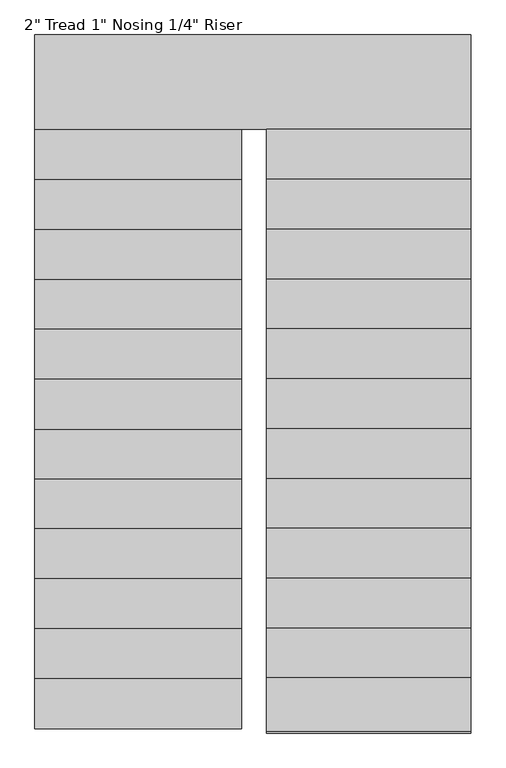
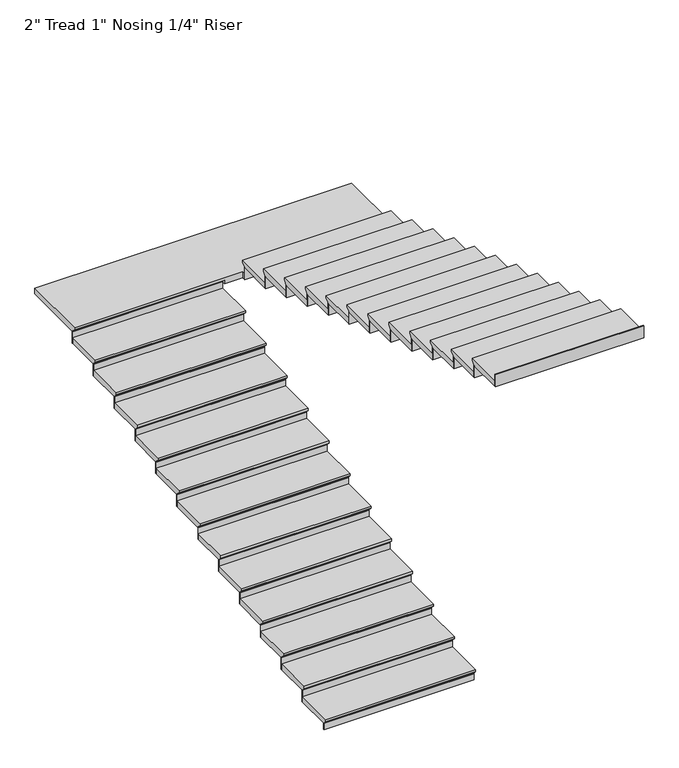
"""IFC4 building model written with IfcOpenShell, lengths in millimetres: stair flight geometry."""

from ifc_helpers import new_model, si_unit, origin, place, context, project, spatial, faceted_brep, source, transform, mapped, element, save


def stair_flight_04159850(model_context):
    return source(origin(), model_context, "Body", "Brep", [
        faceted_brep([(-2593.7381751, -9955.5916506, 12278.4576923), (-2593.7381751, -9955.5916506, 12297.5076923), (-3857.687215, -9955.5916506, 12297.5076923), (-3857.687215, -9955.5916506, 12278.4576923), (-2593.7381751, -9930.1916506, 12253.0576923), (-3857.687215, -9930.1916506, 12253.0576923), (-2593.7381751, -9619.0416506, 12297.5076923), (-3857.687215, -9619.0416506, 12297.5076923), (-3857.687215, -9930.1916506, 12246.7076923), (-3857.687215, -9619.0416506, 12246.7076923), (-2593.7381751, -9619.0416506, 12246.7076923), (-2593.7381751, -9930.1916506, 12246.7076923)], [[[0, 1, 2, 3]], [[4, 0, 3, 5]], [[2, 1, 6, 7]], [[8, 9, 10, 11]], [[2, 7, 9, 8, 5, 3]], [[8, 11, 4, 5]], [[6, 1, 0, 4, 11, 10]], [[7, 6, 10, 9]]]),
        faceted_brep([(-2593.7381751, -9930.1916506, 12246.7076923), (-2593.7381751, -9930.1916506, 12192.0), (-2593.7381751, -9923.8416506, 12192.0), (-2593.7381751, -9923.8416506, 12246.7076923), (-3857.687215, -9930.1916506, 12246.7076923), (-3857.687215, -9923.8416506, 12246.7076923), (-3857.687215, -9923.8416506, 12192.0), (-3857.687215, -9930.1916506, 12192.0)], [[[0, 1, 2, 3]], [[4, 5, 6, 7]], [[1, 0, 4, 7]], [[2, 1, 7, 6]], [[3, 2, 6, 5]], [[0, 3, 5, 4]]]),
        faceted_brep([(-2593.7381751, -9619.0416506, 12352.2153846), (-2593.7381751, -9619.0416506, 12246.7076923), (-2593.7381751, -9612.6916506, 12246.7076923), (-2593.7381751, -9612.6916506, 12352.2153846), (-3857.687215, -9619.0416506, 12352.2153846), (-3857.687215, -9612.6916506, 12352.2153846), (-3857.687215, -9612.6916506, 12246.7076923), (-3857.687215, -9619.0416506, 12246.7076923)], [[[0, 1, 2, 3]], [[4, 5, 6, 7]], [[1, 0, 4, 7]], [[2, 1, 7, 6]], [[3, 2, 6, 5]], [[0, 3, 5, 4]]]),
        faceted_brep([(-3857.687215, -9644.4416506, 12403.0153846), (-2593.7381751, -9644.4416506, 12403.0153846), (-2593.7381751, -9314.2416506, 12403.0153846), (-3857.687215, -9314.2416506, 12403.0153846), (-3857.687215, -9619.0416506, 12352.2153846), (-3857.687215, -9314.2416506, 12352.2153846), (-2593.7381751, -9314.2416506, 12352.2153846), (-2593.7381751, -9619.0416506, 12352.2153846), (-3857.687215, -9619.0416506, 12358.5653846), (-3857.687215, -9644.4416506, 12383.9653846), (-2593.7381751, -9619.0416506, 12358.5653846), (-2593.7381751, -9644.4416506, 12383.9653846)], [[[0, 1, 2, 3]], [[4, 5, 6, 7]], [[0, 3, 5, 4, 8, 9]], [[4, 7, 10, 8]], [[2, 1, 11, 10, 7, 6]], [[3, 2, 6, 5]], [[11, 1, 0, 9]], [[10, 11, 9, 8]]]),
        faceted_brep([(-2593.7381751, -9314.2416506, 12457.7230769), (-2593.7381751, -9314.2416506, 12352.2153846), (-2593.7381751, -9307.8916506, 12352.2153846), (-2593.7381751, -9307.8916506, 12457.7230769), (-3857.687215, -9314.2416506, 12457.7230769), (-3857.687215, -9307.8916506, 12457.7230769), (-3857.687215, -9307.8916506, 12352.2153846), (-3857.687215, -9314.2416506, 12352.2153846)], [[[0, 1, 2, 3]], [[4, 5, 6, 7]], [[1, 0, 4, 7]], [[2, 1, 7, 6]], [[3, 2, 6, 5]], [[0, 3, 5, 4]]]),
        faceted_brep([(-3857.687215, -9339.6416506, 12508.5230769), (-2593.7381751, -9339.6416506, 12508.5230769), (-2593.7381751, -9009.4416506, 12508.5230769), (-3857.687215, -9009.4416506, 12508.5230769), (-3857.687215, -9314.2416506, 12457.7230769), (-3857.687215, -9009.4416506, 12457.7230769), (-2593.7381751, -9009.4416506, 12457.7230769), (-2593.7381751, -9314.2416506, 12457.7230769), (-3857.687215, -9314.2416506, 12464.0730769), (-3857.687215, -9339.6416506, 12489.4730769), (-2593.7381751, -9314.2416506, 12464.0730769), (-2593.7381751, -9339.6416506, 12489.4730769)], [[[0, 1, 2, 3]], [[4, 5, 6, 7]], [[0, 3, 5, 4, 8, 9]], [[4, 7, 10, 8]], [[2, 1, 11, 10, 7, 6]], [[3, 2, 6, 5]], [[11, 1, 0, 9]], [[10, 11, 9, 8]]]),
        faceted_brep([(-2593.7381751, -9009.4416506, 12563.2307692), (-2593.7381751, -9009.4416506, 12457.7230769), (-2593.7381751, -9003.0916506, 12457.7230769), (-2593.7381751, -9003.0916506, 12563.2307692), (-3857.687215, -9009.4416506, 12563.2307692), (-3857.687215, -9003.0916506, 12563.2307692), (-3857.687215, -9003.0916506, 12457.7230769), (-3857.687215, -9009.4416506, 12457.7230769)], [[[0, 1, 2, 3]], [[4, 5, 6, 7]], [[1, 0, 4, 7]], [[2, 1, 7, 6]], [[3, 2, 6, 5]], [[0, 3, 5, 4]]]),
        faceted_brep([(-3857.687215, -9034.8416506, 12614.0307692), (-2593.7381751, -9034.8416506, 12614.0307692), (-2593.7381751, -8704.6416506, 12614.0307692), (-3857.687215, -8704.6416506, 12614.0307692), (-3857.687215, -9009.4416506, 12563.2307692), (-3857.687215, -8704.6416506, 12563.2307692), (-2593.7381751, -8704.6416506, 12563.2307692), (-2593.7381751, -9009.4416506, 12563.2307692), (-3857.687215, -9009.4416506, 12569.5807692), (-3857.687215, -9034.8416506, 12594.9807692), (-2593.7381751, -9009.4416506, 12569.5807692), (-2593.7381751, -9034.8416506, 12594.9807692)], [[[0, 1, 2, 3]], [[4, 5, 6, 7]], [[0, 3, 5, 4, 8, 9]], [[4, 7, 10, 8]], [[2, 1, 11, 10, 7, 6]], [[3, 2, 6, 5]], [[11, 1, 0, 9]], [[10, 11, 9, 8]]]),
        faceted_brep([(-2593.7381751, -8704.6416506, 12668.7384615), (-2593.7381751, -8704.6416506, 12563.2307692), (-2593.7381751, -8698.2916506, 12563.2307692), (-2593.7381751, -8698.2916506, 12668.7384615), (-3857.687215, -8704.6416506, 12668.7384615), (-3857.687215, -8698.2916506, 12668.7384615), (-3857.687215, -8698.2916506, 12563.2307692), (-3857.687215, -8704.6416506, 12563.2307692)], [[[0, 1, 2, 3]], [[4, 5, 6, 7]], [[1, 0, 4, 7]], [[2, 1, 7, 6]], [[3, 2, 6, 5]], [[0, 3, 5, 4]]]),
        faceted_brep([(-3857.687215, -8730.0416506, 12719.5384615), (-2593.7381751, -8730.0416506, 12719.5384615), (-2593.7381751, -8399.8416506, 12719.5384615), (-3857.687215, -8399.8416506, 12719.5384615), (-3857.687215, -8704.6416506, 12668.7384615), (-3857.687215, -8399.8416506, 12668.7384615), (-2593.7381751, -8399.8416506, 12668.7384615), (-2593.7381751, -8704.6416506, 12668.7384615), (-3857.687215, -8704.6416506, 12675.0884615), (-3857.687215, -8730.0416506, 12700.4884615), (-2593.7381751, -8704.6416506, 12675.0884615), (-2593.7381751, -8730.0416506, 12700.4884615)], [[[0, 1, 2, 3]], [[4, 5, 6, 7]], [[0, 3, 5, 4, 8, 9]], [[4, 7, 10, 8]], [[2, 1, 11, 10, 7, 6]], [[3, 2, 6, 5]], [[11, 1, 0, 9]], [[10, 11, 9, 8]]]),
        faceted_brep([(-2593.7381751, -8399.8416506, 12774.2461538), (-2593.7381751, -8399.8416506, 12668.7384615), (-2593.7381751, -8393.4916506, 12668.7384615), (-2593.7381751, -8393.4916506, 12774.2461538), (-3857.687215, -8399.8416506, 12774.2461538), (-3857.687215, -8393.4916506, 12774.2461538), (-3857.687215, -8393.4916506, 12668.7384615), (-3857.687215, -8399.8416506, 12668.7384615)], [[[0, 1, 2, 3]], [[4, 5, 6, 7]], [[1, 0, 4, 7]], [[2, 1, 7, 6]], [[3, 2, 6, 5]], [[0, 3, 5, 4]]]),
        faceted_brep([(-3857.687215, -8425.2416506, 12825.0461538), (-2593.7381751, -8425.2416506, 12825.0461538), (-2593.7381751, -8098.2166506, 12825.0461538), (-3857.687215, -8098.2166506, 12825.0461538), (-3857.687215, -8399.8416506, 12774.2461538), (-3857.687215, -8098.2166506, 12774.2461538), (-2593.7381751, -8098.2166506, 12774.2461538), (-2593.7381751, -8399.8416506, 12774.2461538), (-3857.687215, -8399.8416506, 12780.5961538), (-3857.687215, -8425.2416506, 12805.9961538), (-2593.7381751, -8399.8416506, 12780.5961538), (-2593.7381751, -8425.2416506, 12805.9961538)], [[[0, 1, 2, 3]], [[4, 5, 6, 7]], [[0, 3, 5, 4, 8, 9]], [[4, 7, 10, 8]], [[2, 1, 11, 10, 7, 6]], [[3, 2, 6, 5]], [[11, 1, 0, 9]], [[10, 11, 9, 8]]]),
        faceted_brep([(-2593.7381751, -8098.2166506, 12879.7538462), (-2593.7381751, -8098.2166506, 12774.2461538), (-2593.7381751, -8091.8666506, 12774.2461538), (-2593.7381751, -8091.8666506, 12879.7538462), (-3857.687215, -8098.2166506, 12879.7538462), (-3857.687215, -8091.8666506, 12879.7538462), (-3857.687215, -8091.8666506, 12774.2461538), (-3857.687215, -8098.2166506, 12774.2461538)], [[[0, 1, 2, 3]], [[4, 5, 6, 7]], [[1, 0, 4, 7]], [[2, 1, 7, 6]], [[3, 2, 6, 5]], [[0, 3, 5, 4]]]),
        faceted_brep([(-3857.687215, -8123.6166506, 12930.5538462), (-2593.7381751, -8123.6166506, 12930.5538462), (-2593.7381751, -7790.2416506, 12930.5538462), (-3857.687215, -7790.2416506, 12930.5538462), (-3857.687215, -8098.2166506, 12879.7538462), (-3857.687215, -7790.2416506, 12879.7538462), (-2593.7381751, -7790.2416506, 12879.7538462), (-2593.7381751, -8098.2166506, 12879.7538462), (-3857.687215, -8098.2166506, 12886.1038462), (-3857.687215, -8123.6166506, 12911.5038462), (-2593.7381751, -8098.2166506, 12886.1038462), (-2593.7381751, -8123.6166506, 12911.5038462)], [[[0, 1, 2, 3]], [[4, 5, 6, 7]], [[0, 3, 5, 4, 8, 9]], [[4, 7, 10, 8]], [[2, 1, 11, 10, 7, 6]], [[3, 2, 6, 5]], [[11, 1, 0, 9]], [[10, 11, 9, 8]]]),
        faceted_brep([(-2593.7381751, -7790.2416506, 12985.2615385), (-2593.7381751, -7790.2416506, 12879.7538462), (-2593.7381751, -7783.8916506, 12879.7538462), (-2593.7381751, -7783.8916506, 12985.2615385), (-3857.687215, -7790.2416506, 12985.2615385), (-3857.687215, -7783.8916506, 12985.2615385), (-3857.687215, -7783.8916506, 12879.7538462), (-3857.687215, -7790.2416506, 12879.7538462)], [[[0, 1, 2, 3]], [[4, 5, 6, 7]], [[1, 0, 4, 7]], [[2, 1, 7, 6]], [[3, 2, 6, 5]], [[0, 3, 5, 4]]]),
        faceted_brep([(-3857.687215, -7815.6416506, 13036.0615385), (-2593.7381751, -7815.6416506, 13036.0615385), (-2593.7381751, -7485.4416506, 13036.0615385), (-3857.687215, -7485.4416506, 13036.0615385), (-3857.687215, -7790.2416506, 12985.2615385), (-3857.687215, -7485.4416506, 12985.2615385), (-2593.7381751, -7485.4416506, 12985.2615385), (-2593.7381751, -7790.2416506, 12985.2615385), (-3857.687215, -7790.2416506, 12991.6115385), (-3857.687215, -7815.6416506, 13017.0115385), (-2593.7381751, -7790.2416506, 12991.6115385), (-2593.7381751, -7815.6416506, 13017.0115385)], [[[0, 1, 2, 3]], [[4, 5, 6, 7]], [[0, 3, 5, 4, 8, 9]], [[4, 7, 10, 8]], [[2, 1, 11, 10, 7, 6]], [[3, 2, 6, 5]], [[11, 1, 0, 9]], [[10, 11, 9, 8]]]),
        faceted_brep([(-2593.7381751, -7485.4416506, 13090.7692308), (-2593.7381751, -7485.4416506, 12985.2615385), (-2593.7381751, -7479.0916506, 12985.2615385), (-2593.7381751, -7479.0916506, 13090.7692308), (-3857.687215, -7485.4416506, 13090.7692308), (-3857.687215, -7479.0916506, 13090.7692308), (-3857.687215, -7479.0916506, 12985.2615385), (-3857.687215, -7485.4416506, 12985.2615385)], [[[0, 1, 2, 3]], [[4, 5, 6, 7]], [[1, 0, 4, 7]], [[2, 1, 7, 6]], [[3, 2, 6, 5]], [[0, 3, 5, 4]]]),
        faceted_brep([(-3857.687215, -7510.8416506, 13141.5692308), (-2593.7381751, -7510.8416506, 13141.5692308), (-2593.7381751, -7180.6416506, 13141.5692308), (-3857.687215, -7180.6416506, 13141.5692308), (-3857.687215, -7485.4416506, 13090.7692308), (-3857.687215, -7180.6416506, 13090.7692308), (-2593.7381751, -7180.6416506, 13090.7692308), (-2593.7381751, -7485.4416506, 13090.7692308), (-3857.687215, -7485.4416506, 13097.1192308), (-3857.687215, -7510.8416506, 13122.5192308), (-2593.7381751, -7485.4416506, 13097.1192308), (-2593.7381751, -7510.8416506, 13122.5192308)], [[[0, 1, 2, 3]], [[4, 5, 6, 7]], [[0, 3, 5, 4, 8, 9]], [[4, 7, 10, 8]], [[2, 1, 11, 10, 7, 6]], [[3, 2, 6, 5]], [[11, 1, 0, 9]], [[10, 11, 9, 8]]]),
        faceted_brep([(-2593.7381751, -7180.6416506, 13196.2769231), (-2593.7381751, -7180.6416506, 13090.7692308), (-2593.7381751, -7174.2916506, 13090.7692308), (-2593.7381751, -7174.2916506, 13196.2769231), (-3857.687215, -7180.6416506, 13196.2769231), (-3857.687215, -7174.2916506, 13196.2769231), (-3857.687215, -7174.2916506, 13090.7692308), (-3857.687215, -7180.6416506, 13090.7692308)], [[[0, 1, 2, 3]], [[4, 5, 6, 7]], [[1, 0, 4, 7]], [[2, 1, 7, 6]], [[3, 2, 6, 5]], [[0, 3, 5, 4]]]),
        faceted_brep([(-3857.687215, -7206.0416506, 13247.0769231), (-2593.7381751, -7206.0416506, 13247.0769231), (-2593.7381751, -6875.8416506, 13247.0769231), (-3857.687215, -6875.8416506, 13247.0769231), (-3857.687215, -7180.6416506, 13196.2769231), (-3857.687215, -6875.8416506, 13196.2769231), (-2593.7381751, -6875.8416506, 13196.2769231), (-2593.7381751, -7180.6416506, 13196.2769231), (-3857.687215, -7180.6416506, 13202.6269231), (-3857.687215, -7206.0416506, 13228.0269231), (-2593.7381751, -7180.6416506, 13202.6269231), (-2593.7381751, -7206.0416506, 13228.0269231)], [[[0, 1, 2, 3]], [[4, 5, 6, 7]], [[0, 3, 5, 4, 8, 9]], [[4, 7, 10, 8]], [[2, 1, 11, 10, 7, 6]], [[3, 2, 6, 5]], [[11, 1, 0, 9]], [[10, 11, 9, 8]]]),
        faceted_brep([(-2593.7381751, -6875.8416506, 13301.7846154), (-2593.7381751, -6875.8416506, 13196.2769231), (-2593.7381751, -6869.4916506, 13196.2769231), (-2593.7381751, -6869.4916506, 13301.7846154), (-3857.687215, -6875.8416506, 13301.7846154), (-3857.687215, -6869.4916506, 13301.7846154), (-3857.687215, -6869.4916506, 13196.2769231), (-3857.687215, -6875.8416506, 13196.2769231)], [[[0, 1, 2, 3]], [[4, 5, 6, 7]], [[1, 0, 4, 7]], [[2, 1, 7, 6]], [[3, 2, 6, 5]], [[0, 3, 5, 4]]]),
        faceted_brep([(-3857.687215, -6901.2416506, 13352.5846154), (-2593.7381751, -6901.2416506, 13352.5846154), (-2593.7381751, -6571.0416506, 13352.5846154), (-3857.687215, -6571.0416506, 13352.5846154), (-3857.687215, -6875.8416506, 13301.7846154), (-3857.687215, -6571.0416506, 13301.7846154), (-2593.7381751, -6571.0416506, 13301.7846154), (-2593.7381751, -6875.8416506, 13301.7846154), (-3857.687215, -6875.8416506, 13308.1346154), (-3857.687215, -6901.2416506, 13333.5346154), (-2593.7381751, -6875.8416506, 13308.1346154), (-2593.7381751, -6901.2416506, 13333.5346154)], [[[0, 1, 2, 3]], [[4, 5, 6, 7]], [[0, 3, 5, 4, 8, 9]], [[4, 7, 10, 8]], [[2, 1, 11, 10, 7, 6]], [[3, 2, 6, 5]], [[11, 1, 0, 9]], [[10, 11, 9, 8]]]),
        faceted_brep([(-2593.7381751, -6571.0416506, 13407.2923077), (-2593.7381751, -6571.0416506, 13301.7846154), (-2593.7381751, -6564.6916506, 13301.7846154), (-2593.7381751, -6564.6916506, 13407.2923077), (-3857.687215, -6571.0416506, 13407.2923077), (-3857.687215, -6564.6916506, 13407.2923077), (-3857.687215, -6564.6916506, 13301.7846154), (-3857.687215, -6571.0416506, 13301.7846154)], [[[0, 1, 2, 3]], [[4, 5, 6, 7]], [[1, 0, 4, 7]], [[2, 1, 7, 6]], [[3, 2, 6, 5]], [[0, 3, 5, 4]]]),
        faceted_brep([(-3857.687215, -6596.4416506, 13458.0923077), (-2593.7381751, -6596.4416506, 13458.0923077), (-2593.7381751, -6266.2416506, 13458.0923077), (-3857.687215, -6266.2416506, 13458.0923077), (-3857.687215, -6571.0416506, 13407.2923077), (-3857.687215, -6266.2416506, 13407.2923077), (-2593.7381751, -6266.2416506, 13407.2923077), (-2593.7381751, -6571.0416506, 13407.2923077), (-3857.687215, -6571.0416506, 13413.6423077), (-3857.687215, -6596.4416506, 13439.0423077), (-2593.7381751, -6571.0416506, 13413.6423077), (-2593.7381751, -6596.4416506, 13439.0423077)], [[[0, 1, 2, 3]], [[4, 5, 6, 7]], [[0, 3, 5, 4, 8, 9]], [[4, 7, 10, 8]], [[2, 1, 11, 10, 7, 6]], [[3, 2, 6, 5]], [[11, 1, 0, 9]], [[10, 11, 9, 8]]]),
        faceted_brep([(-2593.7381751, -6266.2416506, 13512.8), (-2593.7381751, -6266.2416506, 13407.2923077), (-2593.7381751, -6259.8916506, 13407.2923077), (-2593.7381751, -6259.8916506, 13512.8), (-3857.687215, -6266.2416506, 13512.8), (-3857.687215, -6259.8916506, 13512.8), (-3857.687215, -6259.8916506, 13407.2923077), (-3857.687215, -6266.2416506, 13407.2923077)], [[[0, 1, 2, 3]], [[4, 5, 6, 7]], [[1, 0, 4, 7]], [[2, 1, 7, 6]], [[3, 2, 6, 5]], [[0, 3, 5, 4]]]),
        faceted_brep([(-1190.687215, -6317.0416506, 13563.6), (-1190.687215, -5713.7916506, 13563.6), (-3857.687215, -5713.7916506, 13563.6), (-3857.687215, -6291.6416506, 13563.6), (-2441.3381751, -6291.6416506, 13563.6), (-2441.3381751, -6317.0416506, 13563.6), (-1190.687215, -5713.7916506, 13512.8), (-1190.687215, -6317.0416506, 13512.8), (-2441.3381751, -6317.0416506, 13512.8), (-2441.3381751, -6291.6416506, 13512.8), (-2593.7381751, -6291.6416506, 13512.8), (-2593.7381751, -6266.2416506, 13512.8), (-3857.687215, -6266.2416506, 13512.8), (-3857.687215, -5713.7916506, 13512.8), (-3857.687215, -6266.2416506, 13519.15), (-3857.687215, -6291.6416506, 13544.55), (-2593.7381751, -6266.2416506, 13519.15), (-2593.7381751, -6291.6416506, 13544.55)], [[[0, 1, 2, 3, 4, 5]], [[6, 7, 8, 9, 10, 11, 12, 13]], [[1, 0, 7, 6]], [[2, 1, 6, 13]], [[3, 2, 13, 12, 14, 15]], [[12, 11, 16, 14]], [[11, 10, 17, 16]], [[4, 3, 15, 17, 10, 9]], [[5, 4, 9, 8]], [[0, 5, 8, 7]], [[15, 14, 16, 17]]]),
        faceted_brep([(-2441.3381751, -6317.0416506, 13618.3076923), (-2441.3381751, -6317.0416506, 13512.8), (-2441.3381751, -6323.3916506, 13512.8), (-2441.3381751, -6323.3916506, 13618.3076923), (-1190.687215, -6317.0416506, 13618.3076923), (-1190.687215, -6323.3916506, 13618.3076923), (-1190.687215, -6323.3916506, 13512.8), (-1190.687215, -6317.0416506, 13512.8)], [[[0, 1, 2, 3]], [[4, 5, 6, 7]], [[1, 0, 4, 7]], [[2, 1, 7, 6]], [[3, 2, 6, 5]], [[0, 3, 5, 4]]]),
        faceted_brep([(-1190.687215, -6291.6416506, 13669.1076923), (-2441.3381751, -6291.6416506, 13669.1076923), (-2441.3381751, -6621.8416506, 13669.1076923), (-1190.687215, -6621.8416506, 13669.1076923), (-1190.687215, -6317.0416506, 13618.3076923), (-1190.687215, -6621.8416506, 13618.3076923), (-2441.3381751, -6621.8416506, 13618.3076923), (-2441.3381751, -6317.0416506, 13618.3076923), (-1190.687215, -6317.0416506, 13624.6576923), (-1190.687215, -6291.6416506, 13650.0576923), (-2441.3381751, -6317.0416506, 13624.6576923), (-2441.3381751, -6291.6416506, 13650.0576923)], [[[0, 1, 2, 3]], [[4, 5, 6, 7]], [[0, 3, 5, 4, 8, 9]], [[4, 7, 10, 8]], [[2, 1, 11, 10, 7, 6]], [[3, 2, 6, 5]], [[11, 1, 0, 9]], [[10, 11, 9, 8]]]),
        faceted_brep([(-2441.3381751, -6621.8416506, 13723.8153846), (-2441.3381751, -6621.8416506, 13618.3076923), (-2441.3381751, -6628.1916506, 13618.3076923), (-2441.3381751, -6628.1916506, 13723.8153846), (-1190.687215, -6621.8416506, 13723.8153846), (-1190.687215, -6628.1916506, 13723.8153846), (-1190.687215, -6628.1916506, 13618.3076923), (-1190.687215, -6621.8416506, 13618.3076923)], [[[0, 1, 2, 3]], [[4, 5, 6, 7]], [[1, 0, 4, 7]], [[2, 1, 7, 6]], [[3, 2, 6, 5]], [[0, 3, 5, 4]]]),
        faceted_brep([(-1190.687215, -6596.4416506, 13774.6153846), (-2441.3381751, -6596.4416506, 13774.6153846), (-2441.3381751, -6926.6416506, 13774.6153846), (-1190.687215, -6926.6416506, 13774.6153846), (-1190.687215, -6621.8416506, 13723.8153846), (-1190.687215, -6926.6416506, 13723.8153846), (-2441.3381751, -6926.6416506, 13723.8153846), (-2441.3381751, -6621.8416506, 13723.8153846), (-1190.687215, -6621.8416506, 13730.1653846), (-1190.687215, -6596.4416506, 13755.5653846), (-2441.3381751, -6621.8416506, 13730.1653846), (-2441.3381751, -6596.4416506, 13755.5653846)], [[[0, 1, 2, 3]], [[4, 5, 6, 7]], [[0, 3, 5, 4, 8, 9]], [[4, 7, 10, 8]], [[2, 1, 11, 10, 7, 6]], [[3, 2, 6, 5]], [[11, 1, 0, 9]], [[10, 11, 9, 8]]]),
        faceted_brep([(-2441.3381751, -6926.6416506, 13829.3230769), (-2441.3381751, -6926.6416506, 13723.8153846), (-2441.3381751, -6932.9916506, 13723.8153846), (-2441.3381751, -6932.9916506, 13829.3230769), (-1190.687215, -6926.6416506, 13829.3230769), (-1190.687215, -6932.9916506, 13829.3230769), (-1190.687215, -6932.9916506, 13723.8153846), (-1190.687215, -6926.6416506, 13723.8153846)], [[[0, 1, 2, 3]], [[4, 5, 6, 7]], [[1, 0, 4, 7]], [[2, 1, 7, 6]], [[3, 2, 6, 5]], [[0, 3, 5, 4]]]),
        faceted_brep([(-1190.687215, -6901.2416506, 13880.1230769), (-2441.3381751, -6901.2416506, 13880.1230769), (-2441.3381751, -7231.4416506, 13880.1230769), (-1190.687215, -7231.4416506, 13880.1230769), (-1190.687215, -6926.6416506, 13829.3230769), (-1190.687215, -7231.4416506, 13829.3230769), (-2441.3381751, -7231.4416506, 13829.3230769), (-2441.3381751, -6926.6416506, 13829.3230769), (-1190.687215, -6926.6416506, 13835.6730769), (-1190.687215, -6901.2416506, 13861.0730769), (-2441.3381751, -6926.6416506, 13835.6730769), (-2441.3381751, -6901.2416506, 13861.0730769)], [[[0, 1, 2, 3]], [[4, 5, 6, 7]], [[0, 3, 5, 4, 8, 9]], [[4, 7, 10, 8]], [[2, 1, 11, 10, 7, 6]], [[3, 2, 6, 5]], [[11, 1, 0, 9]], [[10, 11, 9, 8]]]),
        faceted_brep([(-2441.3381751, -7231.4416506, 13934.8307692), (-2441.3381751, -7231.4416506, 13829.3230769), (-2441.3381751, -7237.7916506, 13829.3230769), (-2441.3381751, -7237.7916506, 13934.8307692), (-1190.687215, -7231.4416506, 13934.8307692), (-1190.687215, -7237.7916506, 13934.8307692), (-1190.687215, -7237.7916506, 13829.3230769), (-1190.687215, -7231.4416506, 13829.3230769)], [[[0, 1, 2, 3]], [[4, 5, 6, 7]], [[1, 0, 4, 7]], [[2, 1, 7, 6]], [[3, 2, 6, 5]], [[0, 3, 5, 4]]]),
        faceted_brep([(-1190.687215, -7206.0416506, 13985.6307692), (-2441.3381751, -7206.0416506, 13985.6307692), (-2441.3381751, -7536.2416506, 13985.6307692), (-1190.687215, -7536.2416506, 13985.6307692), (-1190.687215, -7231.4416506, 13934.8307692), (-1190.687215, -7536.2416506, 13934.8307692), (-2441.3381751, -7536.2416506, 13934.8307692), (-2441.3381751, -7231.4416506, 13934.8307692), (-1190.687215, -7231.4416506, 13941.1807692), (-1190.687215, -7206.0416506, 13966.5807692), (-2441.3381751, -7231.4416506, 13941.1807692), (-2441.3381751, -7206.0416506, 13966.5807692)], [[[0, 1, 2, 3]], [[4, 5, 6, 7]], [[0, 3, 5, 4, 8, 9]], [[4, 7, 10, 8]], [[2, 1, 11, 10, 7, 6]], [[3, 2, 6, 5]], [[11, 1, 0, 9]], [[10, 11, 9, 8]]]),
        faceted_brep([(-2441.3381751, -7536.2416506, 14040.3384615), (-2441.3381751, -7536.2416506, 13934.8307692), (-2441.3381751, -7542.5916506, 13934.8307692), (-2441.3381751, -7542.5916506, 14040.3384615), (-1190.687215, -7536.2416506, 14040.3384615), (-1190.687215, -7542.5916506, 14040.3384615), (-1190.687215, -7542.5916506, 13934.8307692), (-1190.687215, -7536.2416506, 13934.8307692)], [[[0, 1, 2, 3]], [[4, 5, 6, 7]], [[1, 0, 4, 7]], [[2, 1, 7, 6]], [[3, 2, 6, 5]], [[0, 3, 5, 4]]]),
        faceted_brep([(-1190.687215, -7510.8416506, 14091.1384615), (-2441.3381751, -7510.8416506, 14091.1384615), (-2441.3381751, -7841.0416506, 14091.1384615), (-1190.687215, -7841.0416506, 14091.1384615), (-1190.687215, -7536.2416506, 14040.3384615), (-1190.687215, -7841.0416506, 14040.3384615), (-2441.3381751, -7841.0416506, 14040.3384615), (-2441.3381751, -7536.2416506, 14040.3384615), (-1190.687215, -7536.2416506, 14046.6884615), (-1190.687215, -7510.8416506, 14072.0884615), (-2441.3381751, -7536.2416506, 14046.6884615), (-2441.3381751, -7510.8416506, 14072.0884615)], [[[0, 1, 2, 3]], [[4, 5, 6, 7]], [[0, 3, 5, 4, 8, 9]], [[4, 7, 10, 8]], [[2, 1, 11, 10, 7, 6]], [[3, 2, 6, 5]], [[11, 1, 0, 9]], [[10, 11, 9, 8]]]),
        faceted_brep([(-2441.3381751, -7841.0416506, 14145.8461538), (-2441.3381751, -7841.0416506, 14040.3384615), (-2441.3381751, -7847.3916506, 14040.3384615), (-2441.3381751, -7847.3916506, 14145.8461538), (-1190.687215, -7841.0416506, 14145.8461538), (-1190.687215, -7847.3916506, 14145.8461538), (-1190.687215, -7847.3916506, 14040.3384615), (-1190.687215, -7841.0416506, 14040.3384615)], [[[0, 1, 2, 3]], [[4, 5, 6, 7]], [[1, 0, 4, 7]], [[2, 1, 7, 6]], [[3, 2, 6, 5]], [[0, 3, 5, 4]]]),
        faceted_brep([(-1190.687215, -7815.6416506, 14196.6461538), (-2441.3381751, -7815.6416506, 14196.6461538), (-2441.3381751, -8145.8416506, 14196.6461538), (-1190.687215, -8145.8416506, 14196.6461538), (-1190.687215, -7841.0416506, 14145.8461538), (-1190.687215, -8145.8416506, 14145.8461538), (-2441.3381751, -8145.8416506, 14145.8461538), (-2441.3381751, -7841.0416506, 14145.8461538), (-1190.687215, -7841.0416506, 14152.1961538), (-1190.687215, -7815.6416506, 14177.5961538), (-2441.3381751, -7841.0416506, 14152.1961538), (-2441.3381751, -7815.6416506, 14177.5961538)], [[[0, 1, 2, 3]], [[4, 5, 6, 7]], [[0, 3, 5, 4, 8, 9]], [[4, 7, 10, 8]], [[2, 1, 11, 10, 7, 6]], [[3, 2, 6, 5]], [[11, 1, 0, 9]], [[10, 11, 9, 8]]]),
        faceted_brep([(-2441.3381751, -8145.8416506, 14251.3538462), (-2441.3381751, -8145.8416506, 14145.8461538), (-2441.3381751, -8152.1916506, 14145.8461538), (-2441.3381751, -8152.1916506, 14251.3538462), (-1190.687215, -8145.8416506, 14251.3538462), (-1190.687215, -8152.1916506, 14251.3538462), (-1190.687215, -8152.1916506, 14145.8461538), (-1190.687215, -8145.8416506, 14145.8461538)], [[[0, 1, 2, 3]], [[4, 5, 6, 7]], [[1, 0, 4, 7]], [[2, 1, 7, 6]], [[3, 2, 6, 5]], [[0, 3, 5, 4]]]),
        faceted_brep([(-1190.687215, -8120.4416506, 14302.1538462), (-2441.3381751, -8120.4416506, 14302.1538462), (-2441.3381751, -8450.6416506, 14302.1538462), (-1190.687215, -8450.6416506, 14302.1538462), (-1190.687215, -8145.8416506, 14251.3538462), (-1190.687215, -8450.6416506, 14251.3538462), (-2441.3381751, -8450.6416506, 14251.3538462), (-2441.3381751, -8145.8416506, 14251.3538462), (-1190.687215, -8145.8416506, 14257.7038462), (-1190.687215, -8120.4416506, 14283.1038462), (-2441.3381751, -8145.8416506, 14257.7038462), (-2441.3381751, -8120.4416506, 14283.1038462)], [[[0, 1, 2, 3]], [[4, 5, 6, 7]], [[0, 3, 5, 4, 8, 9]], [[4, 7, 10, 8]], [[2, 1, 11, 10, 7, 6]], [[3, 2, 6, 5]], [[11, 1, 0, 9]], [[10, 11, 9, 8]]]),
        faceted_brep([(-2441.3381751, -8450.6416506, 14356.8615385), (-2441.3381751, -8450.6416506, 14251.3538462), (-2441.3381751, -8456.9916506, 14251.3538462), (-2441.3381751, -8456.9916506, 14356.8615385), (-1190.687215, -8450.6416506, 14356.8615385), (-1190.687215, -8456.9916506, 14356.8615385), (-1190.687215, -8456.9916506, 14251.3538462), (-1190.687215, -8450.6416506, 14251.3538462)], [[[0, 1, 2, 3]], [[4, 5, 6, 7]], [[1, 0, 4, 7]], [[2, 1, 7, 6]], [[3, 2, 6, 5]], [[0, 3, 5, 4]]]),
        faceted_brep([(-1190.687215, -8425.2416506, 14407.6615385), (-2441.3381751, -8425.2416506, 14407.6615385), (-2441.3381751, -8755.4416506, 14407.6615385), (-1190.687215, -8755.4416506, 14407.6615385), (-1190.687215, -8450.6416506, 14356.8615385), (-1190.687215, -8755.4416506, 14356.8615385), (-2441.3381751, -8755.4416506, 14356.8615385), (-2441.3381751, -8450.6416506, 14356.8615385), (-1190.687215, -8450.6416506, 14363.2115385), (-1190.687215, -8425.2416506, 14388.6115385), (-2441.3381751, -8450.6416506, 14363.2115385), (-2441.3381751, -8425.2416506, 14388.6115385)], [[[0, 1, 2, 3]], [[4, 5, 6, 7]], [[0, 3, 5, 4, 8, 9]], [[4, 7, 10, 8]], [[2, 1, 11, 10, 7, 6]], [[3, 2, 6, 5]], [[11, 1, 0, 9]], [[10, 11, 9, 8]]]),
        faceted_brep([(-2441.3381751, -8755.4416506, 14462.3692308), (-2441.3381751, -8755.4416506, 14356.8615385), (-2441.3381751, -8761.7916506, 14356.8615385), (-2441.3381751, -8761.7916506, 14462.3692308), (-1190.687215, -8755.4416506, 14462.3692308), (-1190.687215, -8761.7916506, 14462.3692308), (-1190.687215, -8761.7916506, 14356.8615385), (-1190.687215, -8755.4416506, 14356.8615385)], [[[0, 1, 2, 3]], [[4, 5, 6, 7]], [[1, 0, 4, 7]], [[2, 1, 7, 6]], [[3, 2, 6, 5]], [[0, 3, 5, 4]]]),
        faceted_brep([(-1190.687215, -8730.0416506, 14513.1692308), (-2441.3381751, -8730.0416506, 14513.1692308), (-2441.3381751, -9060.2416506, 14513.1692308), (-1190.687215, -9060.2416506, 14513.1692308), (-1190.687215, -8755.4416506, 14462.3692308), (-1190.687215, -9060.2416506, 14462.3692308), (-2441.3381751, -9060.2416506, 14462.3692308), (-2441.3381751, -8755.4416506, 14462.3692308), (-1190.687215, -8755.4416506, 14468.7192308), (-1190.687215, -8730.0416506, 14494.1192308), (-2441.3381751, -8755.4416506, 14468.7192308), (-2441.3381751, -8730.0416506, 14494.1192308)], [[[0, 1, 2, 3]], [[4, 5, 6, 7]], [[0, 3, 5, 4, 8, 9]], [[4, 7, 10, 8]], [[2, 1, 11, 10, 7, 6]], [[3, 2, 6, 5]], [[11, 1, 0, 9]], [[10, 11, 9, 8]]]),
        faceted_brep([(-2441.3381751, -9060.2416506, 14567.8769231), (-2441.3381751, -9060.2416506, 14462.3692308), (-2441.3381751, -9066.5916506, 14462.3692308), (-2441.3381751, -9066.5916506, 14567.8769231), (-1190.687215, -9060.2416506, 14567.8769231), (-1190.687215, -9066.5916506, 14567.8769231), (-1190.687215, -9066.5916506, 14462.3692308), (-1190.687215, -9060.2416506, 14462.3692308)], [[[0, 1, 2, 3]], [[4, 5, 6, 7]], [[1, 0, 4, 7]], [[2, 1, 7, 6]], [[3, 2, 6, 5]], [[0, 3, 5, 4]]]),
        faceted_brep([(-1190.687215, -9034.8416506, 14618.6769231), (-2441.3381751, -9034.8416506, 14618.6769231), (-2441.3381751, -9365.0416506, 14618.6769231), (-1190.687215, -9365.0416506, 14618.6769231), (-1190.687215, -9060.2416506, 14567.8769231), (-1190.687215, -9365.0416506, 14567.8769231), (-2441.3381751, -9365.0416506, 14567.8769231), (-2441.3381751, -9060.2416506, 14567.8769231), (-1190.687215, -9060.2416506, 14574.2269231), (-1190.687215, -9034.8416506, 14599.6269231), (-2441.3381751, -9060.2416506, 14574.2269231), (-2441.3381751, -9034.8416506, 14599.6269231)], [[[0, 1, 2, 3]], [[4, 5, 6, 7]], [[0, 3, 5, 4, 8, 9]], [[4, 7, 10, 8]], [[2, 1, 11, 10, 7, 6]], [[3, 2, 6, 5]], [[11, 1, 0, 9]], [[10, 11, 9, 8]]]),
        faceted_brep([(-2441.3381751, -9365.0416506, 14673.3846154), (-2441.3381751, -9365.0416506, 14567.8769231), (-2441.3381751, -9371.3916506, 14567.8769231), (-2441.3381751, -9371.3916506, 14673.3846154), (-1190.687215, -9365.0416506, 14673.3846154), (-1190.687215, -9371.3916506, 14673.3846154), (-1190.687215, -9371.3916506, 14567.8769231), (-1190.687215, -9365.0416506, 14567.8769231)], [[[0, 1, 2, 3]], [[4, 5, 6, 7]], [[1, 0, 4, 7]], [[2, 1, 7, 6]], [[3, 2, 6, 5]], [[0, 3, 5, 4]]]),
        faceted_brep([(-1190.687215, -9339.6416506, 14724.1846154), (-2441.3381751, -9339.6416506, 14724.1846154), (-2441.3381751, -9669.8416506, 14724.1846154), (-1190.687215, -9669.8416506, 14724.1846154), (-1190.687215, -9365.0416506, 14673.3846154), (-1190.687215, -9669.8416506, 14673.3846154), (-2441.3381751, -9669.8416506, 14673.3846154), (-2441.3381751, -9365.0416506, 14673.3846154), (-1190.687215, -9365.0416506, 14679.7346154), (-1190.687215, -9339.6416506, 14705.1346154), (-2441.3381751, -9365.0416506, 14679.7346154), (-2441.3381751, -9339.6416506, 14705.1346154)], [[[0, 1, 2, 3]], [[4, 5, 6, 7]], [[0, 3, 5, 4, 8, 9]], [[4, 7, 10, 8]], [[2, 1, 11, 10, 7, 6]], [[3, 2, 6, 5]], [[11, 1, 0, 9]], [[10, 11, 9, 8]]]),
        faceted_brep([(-2441.3381751, -9669.8416506, 14778.8923077), (-2441.3381751, -9669.8416506, 14673.3846154), (-2441.3381751, -9676.1916506, 14673.3846154), (-2441.3381751, -9676.1916506, 14778.8923077), (-1190.687215, -9669.8416506, 14778.8923077), (-1190.687215, -9676.1916506, 14778.8923077), (-1190.687215, -9676.1916506, 14673.3846154), (-1190.687215, -9669.8416506, 14673.3846154)], [[[0, 1, 2, 3]], [[4, 5, 6, 7]], [[1, 0, 4, 7]], [[2, 1, 7, 6]], [[3, 2, 6, 5]], [[0, 3, 5, 4]]]),
        faceted_brep([(-2441.3381751, -9974.6416506, 14884.4), (-2441.3381751, -9974.6416506, 14778.8923077), (-2441.3381751, -9980.9916506, 14778.8923077), (-2441.3381751, -9980.9916506, 14884.4), (-1190.687215, -9974.6416506, 14884.4), (-1190.687215, -9980.9916506, 14884.4), (-1190.687215, -9980.9916506, 14778.8923077), (-1190.687215, -9974.6416506, 14778.8923077)], [[[0, 1, 2, 3]], [[4, 5, 6, 7]], [[1, 0, 4, 7]], [[2, 1, 7, 6]], [[3, 2, 6, 5]], [[0, 3, 5, 4]]]),
        faceted_brep([(-1190.687215, -9644.4416506, 14829.6923077), (-2441.3381751, -9644.4416506, 14829.6923077), (-2441.3381751, -9974.6416506, 14829.6923077), (-1190.687215, -9974.6416506, 14829.6923077), (-1190.687215, -9669.8416506, 14778.8923077), (-1190.687215, -9974.6416506, 14778.8923077), (-2441.3381751, -9974.6416506, 14778.8923077), (-2441.3381751, -9669.8416506, 14778.8923077), (-1190.687215, -9669.8416506, 14785.2423077), (-1190.687215, -9644.4416506, 14810.6423077), (-2441.3381751, -9669.8416506, 14785.2423077), (-2441.3381751, -9644.4416506, 14810.6423077)], [[[0, 1, 2, 3]], [[4, 5, 6, 7]], [[0, 3, 5, 4, 8, 9]], [[4, 7, 10, 8]], [[2, 1, 11, 10, 7, 6]], [[3, 2, 6, 5]], [[11, 1, 0, 9]], [[10, 11, 9, 8]]]),
    ])


if __name__ == "__main__":
    model = new_model("IFC4")
    model_context = context("Model", 3, world=origin())
    ifc_project = project(units=[si_unit("LENGTHUNIT", "METRE", prefix="MILLI")], contexts=[model_context])
    site = spatial("IfcSite", under=ifc_project)
    building = spatial("IfcBuilding", under=site)
    placement = place(None, origin())
    stair_flight_shape = stair_flight_04159850(model_context)
    element("IfcStairFlight", 1, ObjectType="2\" Tread 1\" Nosing 1/4\" Riser", at=placement, inside=building, context=model_context, shape_type="MappedRepresentation", body=[
        mapped(stair_flight_shape, transform((0.0, 0.0, 0.0), x_axis=(1.0, 0.0, 0.0), y_axis=(0.0, 1.0, 0.0), z_axis=(0.0, 0.0, 1.0))),
    ])
    save(model, "model.ifc")
